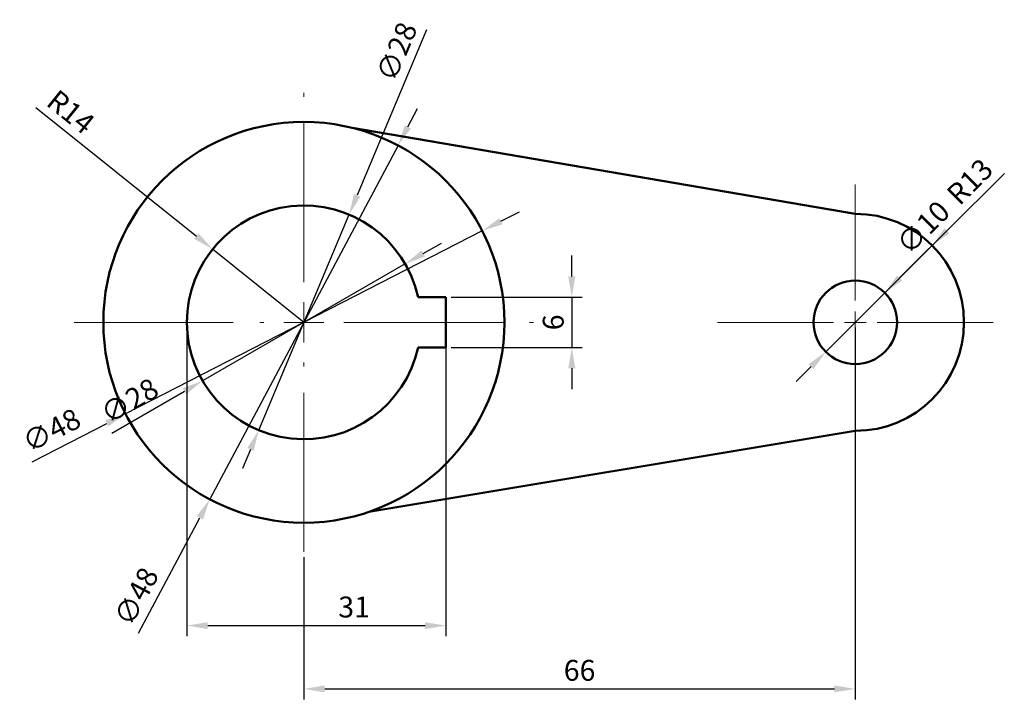
# Model space of a CAD drawing. Units: millimetres. Extents: x 2343 to 2461, y 1495 to 1577.
import ezdxf

# ---------------------------------------------------------------- set-up
doc = ezdxf.new("R2010")
doc.units = ezdxf.units.MM
doc.linetypes.add('CENTER2', pattern=[28.575, 19.05, -3.175, 3.175, -3.175])
doc.linetypes.add('HIDDENX2', pattern=[19.05, 12.7, -6.35])
doc.layers.get('Defpoints').update_dxf_attribs({"color": 3, "linetype": 'HIDDENX2'})
for name, color, linetype, lineweight in [('M-CNTR', 1, 'CENTER2', 18), ('M-DIMS', 2, 'Continuous', 25), ('M-OUTL', 7, 'Continuous', 50)]:
    doc.layers.add(name, color=color, linetype=linetype, lineweight=lineweight)
doc.styles.get("Standard").update_dxf_attribs({"font": 'arial.ttf'})
doc.dimstyles.new('ISO-25', dxfattribs={"dimtxt": 2.5, "dimasz": 2.5, "dimexe": 1.25, "dimexo": 0.625, "dimtad": 1, "dimdec": 0, "dimtxsty": 'Standard', "dimcen": 2.5, "dimadec": 0, "dimazin": 0, "dimtfac": 1, "dimtdec": 0, "dimtmove": 0, "dimatfit": 3, "dimfxl": 1, "dimarcsym": 0})

# ---------------------------------------------------------------- blocks, each defined once
blk = doc.blocks.new('*U1')
at = {"layer": 'M-CNTR', "color": 0, "transparency": 16777216}
for p, q in [((0, 4.8), (0, 27.5)), ((-27.5, 0), (-4.8, 0)), ((4.8, 0), (27.5, 0)), ((0, -27.5), (0, -4.8))]:
    blk.add_line(p, q, dxfattribs=at)
at = {"layer": 'M-CNTR', "color": 0, "linetype": 'Continuous', "transparency": 16777216}
for p, q in [((0, -2.4), (0, 2.4)), ((-2.4, 0), (2.4, 0))]:
    blk.add_line(p, q, dxfattribs=at)
blk = doc.blocks.new('*D3')
at = {"layer": 'Defpoints', "color": 0, "transparency": 16777216}
for p in [(2363.46, 1540.58), (2394.46, 1540.58), (2394.46, 1504.26)]:
    blk.add_point(p, dxfattribs=at)
at = {"layer": 'M-DIMS', "color": 0, "lineweight": -2, "transparency": 16777216}
for p, q in [((2363.46, 1539.96), (2363.46, 1503.01)), ((2394.46, 1539.96), (2394.46, 1503.01)), ((2365.96, 1504.26), (2391.96, 1504.26))]:
    blk.add_line(p, q, dxfattribs=at)
at = {"layer": 'M-DIMS', "color": 0, "transparency": 16777216}
for points in [[(2365.96, 1504.67), (2365.96, 1503.84), (2363.46, 1504.26)], [(2391.96, 1504.67), (2391.96, 1503.84), (2394.46, 1504.26)]]:
    blk.add_solid(points, dxfattribs=at)
at = {"layer": 'M-DIMS', "color": 0, "transparency": 16777216, "insert": (2383.47, 1506.16), "char_height": 2.5, "attachment_point": 5}
blk.add_mtext('31', dxfattribs=at)
blk = doc.blocks.new('*D4')
at = {"layer": 'Defpoints', "color": 0, "transparency": 16777216}
for p in [(2394.46, 1543.58), (2394.46, 1537.58), (2409.53, 1537.58)]:
    blk.add_point(p, dxfattribs=at)
at = {"layer": 'M-DIMS', "color": 0, "lineweight": -2, "transparency": 16777216}
for p, q in [((2409.53, 1546.08), (2409.53, 1548.58)), ((2395.09, 1543.58), (2410.78, 1543.58)), ((2409.53, 1543.58), (2409.53, 1537.58)), ((2395.09, 1537.58), (2410.78, 1537.58)), ((2409.53, 1535.08), (2409.53, 1532.58))]:
    blk.add_line(p, q, dxfattribs=at)
at = {"layer": 'M-DIMS', "color": 0, "transparency": 16777216}
for points in [[(2409.11, 1546.08), (2409.94, 1546.08), (2409.53, 1543.58)], [(2409.11, 1535.08), (2409.94, 1535.08), (2409.53, 1537.58)]]:
    blk.add_solid(points, dxfattribs=at)
at = {"layer": 'M-DIMS', "color": 0, "transparency": 16777216, "insert": (2407.63, 1540.58), "char_height": 2.5, "attachment_point": 5, "rotation": 90}
blk.add_mtext('6', dxfattribs=at)
blk = doc.blocks.new('*D5')
at = {"layer": 'Defpoints', "color": 0, "transparency": 16777216}
for p in [(2366.54, 1549.34), (2377.46, 1540.58)]:
    blk.add_point(p, dxfattribs=at)
at = {"layer": 'M-DIMS', "color": 0, "lineweight": -2, "transparency": 16777216}
for p, q in [((2345.38, 1566.32), (2364.59, 1550.91)), ((2377.46, 1540.58), (2366.54, 1549.34))]:
    blk.add_line(p, q, dxfattribs=at)
at = {"layer": 'M-DIMS', "color": 0, "transparency": 16777216}
blk.add_solid([(2364.85, 1551.23), (2364.33, 1550.58), (2366.54, 1549.34)], dxfattribs=at)
at = {"layer": 'M-DIMS', "color": 0, "transparency": 16777216, "insert": (2349.37, 1565.53), "char_height": 2.5, "attachment_point": 5, "rotation": 321.2571}
blk.add_mtext('R14', dxfattribs=at)
blk = doc.blocks.new('*D6')
at = {"layer": 'Defpoints', "color": 0, "transparency": 16777216}
for p in [(2398.81, 1551.54), (2356.11, 1529.63)]:
    blk.add_point(p, dxfattribs=at)
at = {"layer": 'M-DIMS', "color": 0, "lineweight": -2, "transparency": 16777216}
for p, q in [((2401.04, 1552.68), (2403.26, 1553.82)), ((2398.81, 1551.54), (2356.11, 1529.63)), ((2344.94, 1523.89), (2353.88, 1528.48))]:
    blk.add_line(p, q, dxfattribs=at)
at = {"layer": 'M-DIMS', "color": 0, "transparency": 16777216}
for points in [[(2400.85, 1553.05), (2401.23, 1552.31), (2398.81, 1551.54)], [(2353.69, 1528.86), (2354.07, 1528.11), (2356.11, 1529.63)]]:
    blk.add_solid(points, dxfattribs=at)
at = {"layer": 'M-DIMS', "color": 0, "transparency": 16777216, "insert": (2347.4, 1527.37), "char_height": 2.5, "attachment_point": 5, "rotation": 27.1609}
blk.add_mtext('∅48', dxfattribs=at)
blk = doc.blocks.new('*D7')
at = {"layer": 'Defpoints', "color": 0, "transparency": 16777216}
for p in [(2443.46, 1540.58), (2377.46, 1513.08), (2443.46, 1496.68)]:
    blk.add_point(p, dxfattribs=at)
at = {"layer": 'M-DIMS', "color": 0, "lineweight": -2, "transparency": 16777216}
for p, q in [((2443.46, 1539.96), (2443.46, 1495.43)), ((2377.46, 1512.46), (2377.46, 1495.43)), ((2379.96, 1496.68), (2440.96, 1496.68))]:
    blk.add_line(p, q, dxfattribs=at)
at = {"layer": 'M-DIMS', "color": 0, "transparency": 16777216}
for points in [[(2379.96, 1497.1), (2379.96, 1496.27), (2377.46, 1496.68)], [(2440.96, 1497.1), (2440.96, 1496.27), (2443.46, 1496.68)]]:
    blk.add_solid(points, dxfattribs=at)
at = {"layer": 'M-DIMS', "color": 0, "transparency": 16777216, "insert": (2410.46, 1498.58), "char_height": 2.5, "attachment_point": 5}
blk.add_mtext('66', dxfattribs=at)
blk = doc.blocks.new('*U2')
at = {"layer": 'M-CNTR', "color": 0, "transparency": 16777216}
for p, q in [((0, 2.6), (0, 16.5)), ((-16.5, 0), (-2.6, 0)), ((2.6, 0), (16.5, 0)), ((0, -16.5), (0, -2.6))]:
    blk.add_line(p, q, dxfattribs=at)
at = {"layer": 'M-CNTR', "color": 0, "linetype": 'Continuous', "transparency": 16777216}
for p, q in [((0, -1.3), (0, 1.3)), ((-1.3, 0), (1.3, 0))]:
    blk.add_line(p, q, dxfattribs=at)
blk = doc.blocks.new('*D8')
at = {"layer": 'Defpoints', "color": 0, "transparency": 16777216}
for p in [(2382.88, 1553.49), (2372.05, 1527.67)]:
    blk.add_point(p, dxfattribs=at)
at = {"layer": 'M-DIMS', "color": 0, "lineweight": -2, "transparency": 16777216}
for p, q in [((2392.15, 1575.6), (2383.84, 1555.8)), ((2372.05, 1527.67), (2382.88, 1553.49)), ((2371.08, 1525.37), (2370.11, 1523.06))]:
    blk.add_line(p, q, dxfattribs=at)
at = {"layer": 'M-DIMS', "color": 0, "transparency": 16777216}
for points in [[(2383.46, 1555.96), (2384.23, 1555.64), (2382.88, 1553.49)], [(2370.69, 1525.53), (2371.46, 1525.2), (2372.05, 1527.67)]]:
    blk.add_solid(points, dxfattribs=at)
at = {"layer": 'M-DIMS', "color": 0, "transparency": 16777216, "insert": (2388.87, 1572.87), "char_height": 2.5, "attachment_point": 5, "rotation": 67.2471}
blk.add_mtext('∅28', dxfattribs=at)
blk = doc.blocks.new('*D9')
at = {"layer": 'Defpoints', "color": 0, "transparency": 16777216}
for p in [(2388.73, 1561.77), (2366.19, 1519.39)]:
    blk.add_point(p, dxfattribs=at)
at = {"layer": 'M-DIMS', "color": 0, "lineweight": -2, "transparency": 16777216}
for p, q in [((2389.9, 1563.98), (2391.08, 1566.19)), ((2388.73, 1561.77), (2366.19, 1519.39)), ((2357.66, 1503.34), (2365.02, 1517.18))]:
    blk.add_line(p, q, dxfattribs=at)
at = {"layer": 'M-DIMS', "color": 0, "transparency": 16777216}
for points in [[(2389.53, 1564.18), (2390.27, 1563.78), (2388.73, 1561.77)], [(2364.65, 1517.38), (2365.39, 1516.99), (2366.19, 1519.39)]]:
    blk.add_solid(points, dxfattribs=at)
at = {"layer": 'M-DIMS', "color": 0, "transparency": 16777216, "insert": (2357.69, 1507.6), "char_height": 2.5, "attachment_point": 5, "rotation": 61.9994}
blk.add_mtext('∅48', dxfattribs=at)
blk = doc.blocks.new('*D10')
at = {"layer": 'Defpoints', "color": 0, "transparency": 16777216}
for p in [(2389.59, 1547.58), (2365.34, 1533.58)]:
    blk.add_point(p, dxfattribs=at)
at = {"layer": 'M-DIMS', "color": 0, "lineweight": -2, "transparency": 16777216}
for p, q in [((2391.75, 1548.83), (2393.92, 1550.08)), ((2389.59, 1547.58), (2365.34, 1533.58)), ((2354.46, 1527.3), (2363.17, 1532.33))]:
    blk.add_line(p, q, dxfattribs=at)
at = {"layer": 'M-DIMS', "color": 0, "transparency": 16777216}
for points in [[(2391.54, 1549.19), (2391.96, 1548.47), (2389.59, 1547.58)], [(2362.96, 1532.69), (2363.38, 1531.97), (2365.34, 1533.58)]]:
    blk.add_solid(points, dxfattribs=at)
at = {"layer": 'M-DIMS', "color": 0, "transparency": 16777216, "insert": (2356.75, 1530.9), "char_height": 2.5, "attachment_point": 5, "rotation": 29.998}
blk.add_mtext('∅28', dxfattribs=at)
blk = doc.blocks.new('*D11')
at = {"layer": 'Defpoints', "color": 0, "transparency": 16777216}
for p in [(2452.65, 1549.77), (2443.46, 1540.58)]:
    blk.add_point(p, dxfattribs=at)
at = {"layer": 'M-DIMS', "color": 0, "lineweight": -2, "transparency": 16777216}
for p, q in [((2461.3, 1558.42), (2454.42, 1551.54)), ((2443.46, 1540.58), (2452.65, 1549.77))]:
    blk.add_line(p, q, dxfattribs=at)
at = {"layer": 'M-DIMS', "color": 0, "transparency": 16777216}
blk.add_solid([(2454.13, 1551.84), (2454.71, 1551.25), (2452.65, 1549.77)], dxfattribs=at)
at = {"layer": 'M-DIMS', "color": 0, "transparency": 16777216, "insert": (2457.4, 1557.21), "char_height": 2.5, "attachment_point": 5, "rotation": 45.003}
blk.add_mtext('R13', dxfattribs=at)
blk = doc.blocks.new('*D12')
at = {"layer": 'Defpoints', "color": 0, "transparency": 16777216}
for p in [(2447, 1544.12), (2439.93, 1537.05)]:
    blk.add_point(p, dxfattribs=at)
at = {"layer": 'M-DIMS', "color": 0, "lineweight": -2, "transparency": 16777216}
for p, q in [((2455.86, 1552.99), (2448.76, 1545.89)), ((2439.93, 1537.05), (2447, 1544.12)), ((2438.16, 1535.28), (2436.39, 1533.51))]:
    blk.add_line(p, q, dxfattribs=at)
at = {"layer": 'M-DIMS', "color": 0, "transparency": 16777216}
for points in [[(2448.47, 1546.18), (2449.06, 1545.59), (2447, 1544.12)], [(2437.86, 1535.57), (2438.45, 1534.98), (2439.93, 1537.05)]]:
    blk.add_solid(points, dxfattribs=at)
at = {"layer": 'M-DIMS', "color": 0, "transparency": 16777216, "insert": (2451.8, 1551.71), "char_height": 2.5, "attachment_point": 5, "rotation": 45.0079}
blk.add_mtext('∅10', dxfattribs=at)

msp = doc.modelspace()

# ---------------------------------------------------------------- linework, layer by layer
at = {"layer": 'M-OUTL'}
for p, q in [((2383.25, 1563.87), (2443.46, 1553.58)), ((2391.14, 1543.58), (2394.46, 1543.58)), ((2394.46, 1543.58), (2394.46, 1537.58)), ((2391.14, 1537.58), (2394.46, 1537.58)), ((2385.24, 1517.88), (2443.46, 1527.58))]:
    msp.add_line(p, q, dxfattribs=at)
for centre, radius in [((2377.46, 1540.58), 24), ((2443.46, 1540.58), 5)]:
    msp.add_circle(centre, radius, dxfattribs=at)
for centre, radius, start, end in [((2377.46, 1540.58), 14, 12.3736, 347.6264), ((2443.46, 1540.58), 13, 270, 90)]:
    msp.add_arc(centre, radius, start, end, dxfattribs=at)

# ---------------------------------------------------------------- block references
at = {"layer": 'M-CNTR'}
for name, p in [('*U1', (2377.46, 1540.58)), ('*U2', (2443.46, 1540.58))]:
    msp.add_blockref(name, p, dxfattribs=at)

# ---------------------------------------------------------------- dimensions: what is measured, and where the dimension line sits
at = {"layer": 'M-DIMS'}
for p1, p2, override, picture, middle in [((2372.05, 1527.67), (2382.88, 1553.49), {"dimclrd": 0, "dimclre": 0, "dimclrt": 0}, '*D8', (2390.68, 1572.11)), ((2388.73, 1561.77), (2366.19, 1519.39), {"dimdec": 0, "dimlfac": 1, "dimrnd": 0, "dimzin": 0, "dimdsep": 46, "dimlunit": 2}, '*D9', (2359.43, 1506.68)), ((2439.93, 1537.05), (2447, 1544.12), {"dimdec": 0, "dimlfac": 1, "dimrnd": 0, "dimzin": 0, "dimdsep": 46, "dimlunit": 2}, '*D12', (2453.2, 1550.32)), ((2389.59, 1547.58), (2365.34, 1533.58), {"dimdec": 0, "dimlfac": 1, "dimrnd": 0, "dimzin": 0, "dimdsep": 46, "dimlunit": 2}, '*D10', (2357.73, 1529.19))]:
    dim = msp.add_diameter_dim_2p(p1=p1, p2=p2, dimstyle='ISO-25', override=override, dxfattribs=at)
    dim.commit()
    dim.dimension.update_dxf_attribs({"geometry": picture, "text_midpoint": middle, "dimtype": 163})
dim = msp.add_radius_dim(center=(2377.46, 1540.58), mpoint=(2366.54, 1549.34), dimstyle='ISO-25', override={"dimclrd": 0, "dimclre": 0, "dimclrt": 0}, dxfattribs=at)
dim.commit()
dim.dimension.update_dxf_attribs({"geometry": '*D5', "text_midpoint": (2348.19, 1564.07), "dimtype": 164})
dim = msp.add_radius_dim(center=(2443.46, 1540.58), mpoint=(2452.65, 1549.77), dimstyle='ISO-25', override={"dimdec": 0, "dimlfac": 1, "dimrnd": 0, "dimzin": 0, "dimdsep": 46, "dimlunit": 2}, dxfattribs=at)
dim.commit()
dim.dimension.update_dxf_attribs({"geometry": '*D11', "text_midpoint": (2457.4, 1557.21)})
dim = msp.add_diameter_dim_2p(p1=(2398.81, 1551.54), p2=(2356.11, 1529.63), dimstyle='ISO-25', override={"dimclrd": 0, "dimclre": 0, "dimclrt": 0}, dxfattribs=at)
dim.commit()
dim.dimension.update_dxf_attribs({"geometry": '*D6', "text_midpoint": (2347.4, 1527.37)})
dim = msp.add_linear_dim(base=(2409.53, 1537.58), p1=(2394.46, 1543.58), p2=(2394.46, 1537.58), angle=90, dimstyle='ISO-25', override={"dimclrd": 0, "dimclre": 0, "dimclrt": 0}, dxfattribs=at)
dim.commit()
dim.dimension.update_dxf_attribs({"geometry": '*D4', "text_midpoint": (2407.63, 1540.58)})
dim = msp.add_linear_dim(base=(2394.46, 1504.26), p1=(2363.46, 1540.58), p2=(2394.46, 1540.58), dimstyle='ISO-25', override={"dimclrd": 0, "dimclre": 0, "dimclrt": 0}, dxfattribs=at)
dim.commit()
dim.dimension.update_dxf_attribs({"geometry": '*D3', "text_midpoint": (2383.47, 1504.26), "dimtype": 160})
dim = msp.add_linear_dim(base=(2443.46, 1496.68), p1=(2377.46, 1513.08), p2=(2443.46, 1540.58), dimstyle='ISO-25', override={"dimclrd": 0, "dimclre": 0, "dimclrt": 0}, dxfattribs=at)
dim.commit()
dim.dimension.update_dxf_attribs({"geometry": '*D7', "text_midpoint": (2410.46, 1498.58)})

doc.saveas('drawing.dxf')
